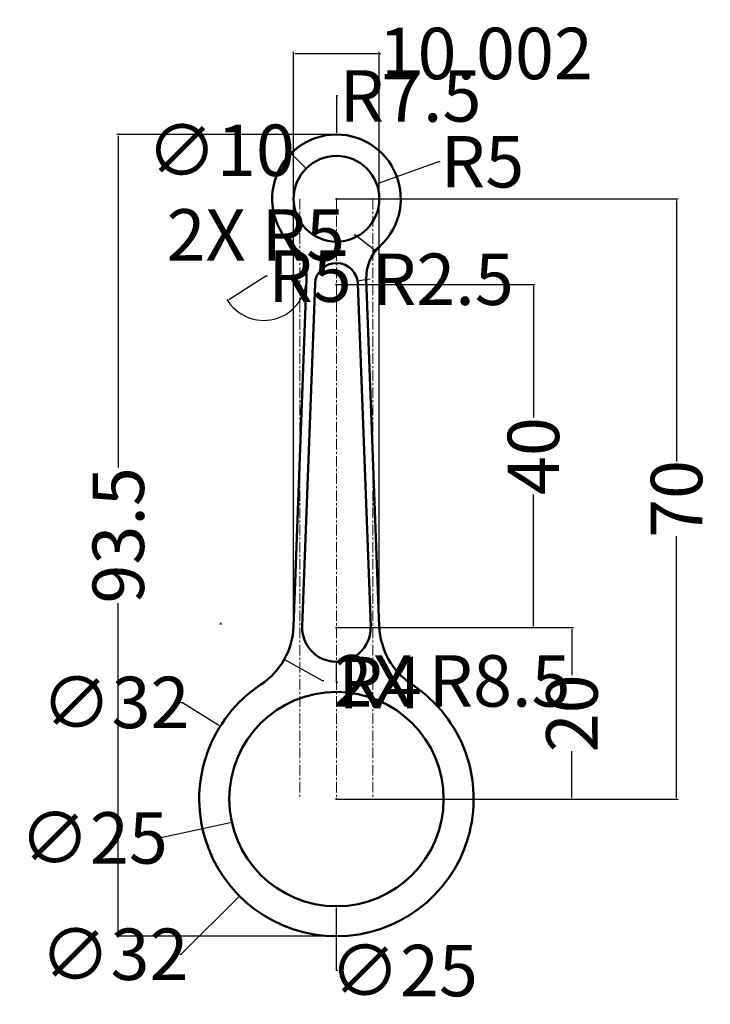
# Model space of a CAD drawing. Units: millimetres. Extents: x 20 to 101, y -5 to 109.
import ezdxf

# ---------------------------------------------------------------- set-up
doc = ezdxf.new("R2010")
doc.units = ezdxf.units.MM
doc.header["$MEASUREMENT"] = 0
doc.linetypes.add('CENTER', pattern=[2, 1.25, -0.25, 0.25, -0.25])
for name, color, linetype, lineweight in [('M-CNTR', 4, 'CENTER', 18), ('M-DIMS', 2, 'Continuous', 25), ('M-OUTL', 7, 'Continuous', 50)]:
    doc.layers.add(name, color=color, linetype=linetype, lineweight=lineweight)
doc.styles.get("Standard").update_dxf_attribs({"font": 'arial.ttf'})
doc.dimstyles.get("Standard").update_dxf_attribs({"dimtxt": 6, "dimasz": 0.18, "dimexe": 0.18, "dimexo": 0.0625, "dimgap": 0.09, "dimtad": 0, "dimtoh": 1, "dimdec": 0, "dimzin": 0, "dimdsep": 46, "dimtxsty": 'Standard', "dimcen": 0.09, "dimadec": 0, "dimazin": 0, "dimtfac": 1, "dimtdec": 0, "dimtofl": 0, "dimtmove": 0, "dimatfit": 3, "dimfxl": 1, "dimtolj": 1, "dimtzin": 0, "dimarcsym": 0})

# ---------------------------------------------------------------- blocks, each defined once
blk = doc.blocks.new('*D1')
at = {"layer": 'Defpoints', "color": 0, "transparency": 16777216}
for p in [(57.38, 78.56), (57.38, 38.56), (80.35, 38.56)]:
    blk.add_point(p, dxfattribs=at)
at = {"layer": 'M-DIMS', "color": 0, "lineweight": -2, "transparency": 16777216}
for p, q in [((57.44, 78.56), (80.53, 78.56)), ((80.35, 78.38), (80.35, 63.06)), ((80.35, 38.74), (80.35, 54.06)), ((57.44, 38.56), (80.53, 38.56))]:
    blk.add_line(p, q, dxfattribs=at)
at = {"layer": 'M-DIMS', "color": 0, "transparency": 16777216}
for points in [[(80.32, 78.38), (80.38, 78.38), (80.35, 78.56)], [(80.32, 38.74), (80.38, 38.74), (80.35, 38.56)]]:
    blk.add_solid(points, dxfattribs=at)
at = {"layer": 'M-DIMS', "color": 0, "transparency": 16777216, "insert": (80.35, 58.56), "char_height": 6, "attachment_point": 5, "rotation": 90}
blk.add_mtext('\\A1;40', dxfattribs=at)
blk = doc.blocks.new('*D2')
at = {"layer": 'Defpoints', "color": 0, "transparency": 16777216}
for p in [(57.38, 38.56), (57.38, 18.56), (84.84, 18.56)]:
    blk.add_point(p, dxfattribs=at)
at = {"layer": 'M-DIMS', "color": 0, "lineweight": -2, "transparency": 16777216}
for p, q in [((57.44, 38.56), (85.02, 38.56)), ((84.84, 38.38), (84.84, 32.99)), ((84.84, 18.74), (84.84, 24.13)), ((57.44, 18.56), (85.02, 18.56))]:
    blk.add_line(p, q, dxfattribs=at)
at = {"layer": 'M-DIMS', "color": 0, "transparency": 16777216}
for points in [[(84.81, 38.38), (84.87, 38.38), (84.84, 38.56)], [(84.81, 18.74), (84.87, 18.74), (84.84, 18.56)]]:
    blk.add_solid(points, dxfattribs=at)
at = {"layer": 'M-DIMS', "color": 0, "transparency": 16777216, "insert": (84.84, 28.56), "char_height": 6, "attachment_point": 5, "rotation": 90}
blk.add_mtext('\\A1;20', dxfattribs=at)
blk = doc.blocks.new('*D3')
at = {"layer": 'Defpoints', "color": 0, "transparency": 16777216}
for p in [(57.38, 88.56), (57.38, 18.56), (97.04, 18.56)]:
    blk.add_point(p, dxfattribs=at)
at = {"layer": 'M-DIMS', "color": 0, "lineweight": -2, "transparency": 16777216}
for p, q in [((57.44, 88.56), (97.22, 88.56)), ((97.04, 88.38), (97.04, 57.91)), ((97.04, 18.74), (97.04, 49.21)), ((57.44, 18.56), (97.22, 18.56))]:
    blk.add_line(p, q, dxfattribs=at)
at = {"layer": 'M-DIMS', "color": 0, "transparency": 16777216}
for points in [[(97.01, 88.38), (97.07, 88.38), (97.04, 88.56)], [(97.01, 18.74), (97.07, 18.74), (97.04, 18.56)]]:
    blk.add_solid(points, dxfattribs=at)
at = {"layer": 'M-DIMS', "color": 0, "transparency": 16777216, "insert": (97.04, 53.56), "char_height": 6, "attachment_point": 5, "rotation": 90}
blk.add_mtext('\\A1;70', dxfattribs=at)
blk = doc.blocks.new('*D4')
at = {"layer": 'Defpoints', "color": 0, "transparency": 16777216}
for p in [(48.9, 79.38), (44.7, 76.67)]:
    blk.add_point(p, dxfattribs=at)
at = {"layer": 'M-DIMS', "color": 0, "lineweight": -2, "transparency": 16777216}
for p, q in [((49.16, 79.54), (44.85, 76.77)), ((49.34, 79.54), (49.16, 79.54))]:
    blk.add_line(p, q, dxfattribs=at)
blk.add_arc((48.9, 79.38), 5, 210.6462, 357.1347, dxfattribs=at)
at = {"layer": 'M-DIMS', "color": 0, "transparency": 16777216}
blk.add_solid([(44.83, 76.8), (44.86, 76.75), (44.7, 76.67)], dxfattribs=at)
at = {"layer": 'M-DIMS', "color": 0, "transparency": 16777216, "insert": (54.29, 79.54), "char_height": 6, "attachment_point": 5}
blk.add_mtext('\\A1;R5', dxfattribs=at)
blk = doc.blocks.new('*D5')
at = {"layer": 'Defpoints', "color": 0, "transparency": 16777216}
for p in [(62.08, 90.27), (57.38, 88.56)]:
    blk.add_point(p, dxfattribs=at)
at = {"layer": 'M-DIMS', "color": 0, "lineweight": -2, "transparency": 16777216}
for p, q in [((69.28, 92.88), (62.25, 90.33)), ((69.46, 92.88), (69.28, 92.88)), ((57.29, 88.56), (57.47, 88.56)), ((57.38, 88.47), (57.38, 88.65))]:
    blk.add_line(p, q, dxfattribs=at)
at = {"layer": 'M-DIMS', "color": 0, "transparency": 16777216}
blk.add_solid([(62.24, 90.36), (62.26, 90.3), (62.08, 90.27)], dxfattribs=at)
at = {"layer": 'M-DIMS', "color": 0, "transparency": 16777216, "insert": (74.41, 92.88), "char_height": 6, "attachment_point": 5}
blk.add_mtext('\\A1;R5', dxfattribs=at)
blk = doc.blocks.new('*D6')
at = {"layer": 'Defpoints', "color": 0, "transparency": 16777216}
for p in [(43.83, 27.06), (70.94, 10.06)]:
    blk.add_point(p, dxfattribs=at)
at = {"layer": 'M-DIMS', "color": 0, "lineweight": -2, "transparency": 16777216}
for p, q in [((39.23, 29.83), (39.41, 29.83)), ((39.41, 29.83), (43.67, 27.16)), ((57.29, 18.56), (57.47, 18.56)), ((57.38, 18.47), (57.38, 18.65))]:
    blk.add_line(p, q, dxfattribs=at)
at = {"layer": 'M-DIMS', "color": 0, "transparency": 16777216}
blk.add_solid([(43.69, 27.18), (43.66, 27.13), (43.83, 27.06)], dxfattribs=at)
at = {"layer": 'M-DIMS', "color": 0, "transparency": 16777216, "insert": (31.61, 29.83), "char_height": 6, "attachment_point": 5}
blk.add_mtext('\\A1;∅32', dxfattribs=at)
blk = doc.blocks.new('*D7')
at = {"layer": 'Defpoints', "color": 0, "transparency": 16777216}
for p in [(69.59, 21.24), (45.17, 15.88)]:
    blk.add_point(p, dxfattribs=at)
at = {"layer": 'M-DIMS', "color": 0, "lineweight": -2, "transparency": 16777216}
for p, q in [((57.29, 18.56), (57.47, 18.56)), ((57.38, 18.47), (57.38, 18.65)), ((36.75, 14.03), (45, 15.84))]:
    blk.add_line(p, q, dxfattribs=at)
at = {"layer": 'M-DIMS', "color": 0, "transparency": 16777216}
blk.add_solid([(44.99, 15.87), (45, 15.81), (45.17, 15.88)], dxfattribs=at)
at = {"layer": 'M-DIMS', "color": 0, "transparency": 16777216, "insert": (29.08, 14.03), "char_height": 6, "attachment_point": 5}
blk.add_mtext('\\A1;∅25', dxfattribs=at)
blk = doc.blocks.new('*D8')
at = {"layer": 'Defpoints', "color": 0, "transparency": 16777216}
for p in [(31.94, 96.06), (57.38, 96.06), (57.38, 2.56)]:
    blk.add_point(p, dxfattribs=at)
at = {"layer": 'M-DIMS', "color": 0, "lineweight": -2, "transparency": 16777216}
for p, q in [((57.32, 96.06), (31.76, 96.06)), ((31.94, 95.88), (31.94, 57.22)), ((31.94, 2.74), (31.94, 41.41)), ((57.32, 2.56), (31.76, 2.56))]:
    blk.add_line(p, q, dxfattribs=at)
at = {"layer": 'M-DIMS', "color": 0, "transparency": 16777216}
for points in [[(31.91, 95.88), (31.97, 95.88), (31.94, 96.06)], [(31.91, 2.74), (31.97, 2.74), (31.94, 2.56)]]:
    blk.add_solid(points, dxfattribs=at)
at = {"layer": 'M-DIMS', "color": 0, "transparency": 16777216, "insert": (31.94, 49.31), "char_height": 6, "attachment_point": 5, "rotation": 90}
blk.add_mtext('\\A1;93.5', dxfattribs=at)
blk = doc.blocks.new('*D9')
at = {"layer": 'Defpoints', "color": 0, "transparency": 16777216}
for p in [(62.38, 105.51), (52.38, 38.69), (62.38, 38.69)]:
    blk.add_point(p, dxfattribs=at)
at = {"layer": 'M-DIMS', "color": 0, "lineweight": -2, "transparency": 16777216}
for p, q in [((52.38, 38.75), (52.38, 105.69)), ((62.38, 38.75), (62.38, 105.69)), ((52.56, 105.51), (62.2, 105.51)), ((62.38, 105.51), (62.56, 105.51))]:
    blk.add_line(p, q, dxfattribs=at)
at = {"layer": 'M-DIMS', "color": 0, "transparency": 16777216}
for points in [[(52.56, 105.54), (52.56, 105.48), (52.38, 105.51)], [(62.2, 105.54), (62.2, 105.48), (62.38, 105.51)]]:
    blk.add_solid(points, dxfattribs=at)
at = {"layer": 'M-DIMS', "color": 0, "transparency": 16777216, "insert": (74.79, 105.51), "char_height": 6, "attachment_point": 5}
blk.add_mtext('\\A1;10.002', dxfattribs=at)
blk = doc.blocks.new('*D10')
at = {"layer": 'Defpoints', "color": 0, "transparency": 16777216}
for p in [(68.69, 29.88), (46.07, 7.25)]:
    blk.add_point(p, dxfattribs=at)
at = {"layer": 'M-DIMS', "color": 0, "lineweight": -2, "transparency": 16777216}
for p, q in [((57.29, 18.56), (57.47, 18.56)), ((57.38, 18.47), (57.38, 18.65)), ((39.28, 0.46), (45.94, 7.12)), ((39.1, 0.46), (39.28, 0.46))]:
    blk.add_line(p, q, dxfattribs=at)
at = {"layer": 'M-DIMS', "color": 0, "transparency": 16777216}
blk.add_solid([(45.92, 7.14), (45.96, 7.1), (46.07, 7.25)], dxfattribs=at)
at = {"layer": 'M-DIMS', "color": 0, "transparency": 16777216, "insert": (31.48, 0.46), "char_height": 6, "attachment_point": 5}
blk.add_mtext('\\A1;∅32', dxfattribs=at)
blk = doc.blocks.new('*D11')
at = {"layer": 'Defpoints', "color": 0, "transparency": 16777216}
for p in [(57.38, 31.06), (57.38, 6.06)]:
    blk.add_point(p, dxfattribs=at)
at = {"layer": 'M-DIMS', "color": 0, "lineweight": -2, "transparency": 16777216}
for p, q in [((57.29, 18.56), (57.47, 18.56)), ((57.38, 18.47), (57.38, 18.65)), ((57.38, -1.44), (57.38, 5.88)), ((57.56, -1.44), (57.38, -1.44))]:
    blk.add_line(p, q, dxfattribs=at)
at = {"layer": 'M-DIMS', "color": 0, "transparency": 16777216}
blk.add_solid([(57.41, 5.88), (57.35, 5.88), (57.38, 6.06)], dxfattribs=at)
at = {"layer": 'M-DIMS', "color": 0, "transparency": 16777216, "insert": (65.24, -1.44), "char_height": 6, "attachment_point": 5}
blk.add_mtext('\\A1;∅25', dxfattribs=at)
blk = doc.blocks.new('*D12')
at = {"layer": 'Defpoints', "color": 0, "transparency": 16777216}
for p in [(43.89, 39.01), (51.29, 34.84)]:
    blk.add_point(p, dxfattribs=at)
at = {"layer": 'M-DIMS', "color": 0, "lineweight": -2, "transparency": 16777216}
for p, q in [((43.89, 38.92), (43.89, 39.1)), ((43.8, 39.01), (43.98, 39.01)), ((55.74, 32.34), (51.45, 34.75)), ((55.92, 32.34), (55.74, 32.34))]:
    blk.add_line(p, q, dxfattribs=at)
at = {"layer": 'M-DIMS', "color": 0, "transparency": 16777216}
blk.add_solid([(51.47, 34.78), (51.44, 34.73), (51.29, 34.84)], dxfattribs=at)
at = {"layer": 'M-DIMS', "color": 0, "transparency": 16777216, "insert": (70.86, 32.34), "char_height": 6, "attachment_point": 5}
blk.add_mtext('\\A1;2X R8.5', dxfattribs=at)
blk = doc.blocks.new('*D13')
at = {"layer": 'Defpoints', "color": 0, "transparency": 16777216}
for p in [(57.38, 96.06), (57.38, 88.56)]:
    blk.add_point(p, dxfattribs=at)
at = {"layer": 'M-DIMS', "color": 0, "lineweight": -2, "transparency": 16777216}
for p, q in [((57.56, 100.56), (57.38, 100.56)), ((57.38, 100.56), (57.38, 96.24)), ((57.29, 88.56), (57.47, 88.56)), ((57.38, 88.47), (57.38, 88.65))]:
    blk.add_line(p, q, dxfattribs=at)
at = {"layer": 'M-DIMS', "color": 0, "transparency": 16777216}
blk.add_solid([(57.35, 96.24), (57.41, 96.24), (57.38, 96.06)], dxfattribs=at)
at = {"layer": 'M-DIMS', "color": 0, "transparency": 16777216, "insert": (66.01, 100.56), "char_height": 6, "attachment_point": 5}
blk.add_mtext('\\A1;R7.5', dxfattribs=at)
blk = doc.blocks.new('*D14')
at = {"layer": 'Defpoints', "color": 0, "transparency": 16777216}
for p in [(53.85, 92.1), (60.92, 85.03)]:
    blk.add_point(p, dxfattribs=at)
at = {"layer": 'M-DIMS', "color": 0, "lineweight": -2, "transparency": 16777216}
for p, q in [((51.54, 94.22), (51.72, 94.22)), ((51.72, 94.22), (53.72, 92.23)), ((57.29, 88.56), (57.47, 88.56)), ((57.38, 88.47), (57.38, 88.65))]:
    blk.add_line(p, q, dxfattribs=at)
at = {"layer": 'M-DIMS', "color": 0, "transparency": 16777216}
blk.add_solid([(53.74, 92.25), (53.7, 92.2), (53.85, 92.1)], dxfattribs=at)
at = {"layer": 'M-DIMS', "color": 0, "transparency": 16777216, "insert": (43.9, 94.22), "char_height": 6, "attachment_point": 5}
blk.add_mtext('\\A1;∅10', dxfattribs=at)
blk = doc.blocks.new('*D15')
at = {"layer": 'Defpoints', "color": 0, "transparency": 16777216}
for p in [(61.94, 82.49), (65.86, 79.38)]:
    blk.add_point(p, dxfattribs=at)
at = {"layer": 'M-DIMS', "color": 0, "lineweight": -2, "transparency": 16777216}
for p, q in [((59.41, 84.35), (59.59, 84.35)), ((59.59, 84.35), (61.8, 82.6)), ((65.77, 79.38), (65.95, 79.38)), ((65.86, 79.29), (65.86, 79.47))]:
    blk.add_line(p, q, dxfattribs=at)
at = {"layer": 'M-DIMS', "color": 0, "transparency": 16777216}
blk.add_solid([(61.82, 82.62), (61.78, 82.58), (61.94, 82.49)], dxfattribs=at)
at = {"layer": 'M-DIMS', "color": 0, "transparency": 16777216, "insert": (47.97, 84.35), "char_height": 6, "attachment_point": 5}
blk.add_mtext('\\A1;2X R5', dxfattribs=at)
blk = doc.blocks.new('*D16')
at = {"layer": 'Defpoints', "color": 0, "transparency": 16777216}
for p in [(57.38, 38.56), (57.38, 34.56)]:
    blk.add_point(p, dxfattribs=at)
at = {"layer": 'M-DIMS', "color": 0, "lineweight": -2, "transparency": 16777216}
for p, q in [((57.29, 38.56), (57.47, 38.56)), ((57.38, 38.47), (57.38, 38.65)), ((57.38, 32.16), (57.38, 34.38)), ((57.56, 32.16), (57.38, 32.16))]:
    blk.add_line(p, q, dxfattribs=at)
at = {"layer": 'M-DIMS', "color": 0, "transparency": 16777216}
blk.add_solid([(57.41, 34.38), (57.35, 34.38), (57.38, 34.56)], dxfattribs=at)
at = {"layer": 'M-DIMS', "color": 0, "transparency": 16777216, "insert": (62.48, 32.16), "char_height": 6, "attachment_point": 5}
blk.add_mtext('\\A1;R4', dxfattribs=at)
blk = doc.blocks.new('*D17')
at = {"layer": 'Defpoints', "color": 0, "transparency": 16777216}
for p in [(57.38, 78.56), (59.85, 78.95)]:
    blk.add_point(p, dxfattribs=at)
at = {"layer": 'M-DIMS', "color": 0, "lineweight": -2, "transparency": 16777216}
for p, q in [((57.29, 78.56), (57.47, 78.56)), ((57.38, 78.47), (57.38, 78.65)), ((61.33, 79.18), (60.03, 78.98))]:
    blk.add_line(p, q, dxfattribs=at)
at = {"layer": 'M-DIMS', "color": 0, "transparency": 16777216}
blk.add_solid([(60.02, 79.01), (60.03, 78.95), (59.85, 78.95)], dxfattribs=at)
at = {"layer": 'M-DIMS', "color": 0, "transparency": 16777216, "insert": (69.78, 79.18), "char_height": 6, "attachment_point": 5}
blk.add_mtext('\\A1;R2.5', dxfattribs=at)

msp = doc.modelspace()

# ---------------------------------------------------------------- linework, layer by layer
at = {"layer": 'M-CNTR'}
for p, q in [((53.1307, 88.5622), (53.1307, 18.5622)), ((57.3807, 88.5622), (57.3807, 18.5622)), ((61.6307, 88.5622), (61.6307, 18.5622))]:
    msp.add_line(p, q, dxfattribs=at)
at = {"layer": 'M-OUTL'}
for p, q in [((53.8995, 79.1889), (52.3798, 38.6918)), ((54.8825, 78.6559), (53.3836, 38.7122)), ((59.879, 78.6559), (61.3779, 38.7122)), ((60.862, 79.1889), (62.3817, 38.6918))]:
    msp.add_line(p, q, dxfattribs=at)
for centre, radius in [((57.3807, 88.5622), 5), ((57.3807, 18.5622), 12.5)]:
    msp.add_circle(centre, radius, dxfattribs=at)
for centre, radius, start, end in [((57.3807, 88.5622), 7.5, 304.518108, 235.481892), ((48.903, 79.3764), 5, 357.850904, 47.295513), ((65.8585, 79.3764), 5, 132.704487, 182.149096), ((57.3807, 78.5622), 2.5, 0, 177.850904), ((43.8858, 39.0106), 8.5, 303.422933, 357.850904), ((57.3807, 38.5622), 4, 177.850904, 2.149096), ((70.8757, 39.0106), 8.5, 182.149096, 236.577067), ((57.3807, 18.5622), 16, 123.422933, 56.577067)]:
    msp.add_arc(centre, radius, start, end, dxfattribs=at)

# ---------------------------------------------------------------- dimensions: what is measured, and where the dimension line sits
at = {"layer": 'M-DIMS'}
dim = msp.add_linear_dim(base=(62.3817, 105.5122), p1=(52.3798, 38.6918), p2=(62.3817, 38.6918), dimstyle='Standard', override={"dimdec": 3, "dimlfac": 1, "dimrnd": 0, "dimzin": 0, "dimdsep": 46, "dimlunit": 2}, dxfattribs=at)
dim.commit()
dim.dimension.update_dxf_attribs({"geometry": '*D9', "text_midpoint": (74.7929, 105.5122)})
for center, mpoint, override, picture, middle in [((57.3807, 88.5622), (57.381, 96.0622), {"dimdec": 1, "dimlfac": 1, "dimrnd": 0, "dimzin": 0, "dimdsep": 46, "dimlunit": 2}, '*D13', (66.0065, 100.5622)), ((57.3807, 88.5622), (62.0805, 90.2689), {"dimclrd": 0, "dimclre": 0, "dimclrt": 0}, '*D5', (74.4096, 92.8831)), ((48.903, 79.3764), (44.6959, 76.6746), {"dimclrd": 0, "dimclre": 0, "dimclrt": 0}, '*D4', (54.2942, 79.544)), ((57.3807, 78.5622), (59.8505, 78.9501), {"dimdec": 1, "dimlfac": 1, "dimrnd": 0, "dimzin": 0, "dimdsep": 46, "dimlunit": 2}, '*D17', (61.3323, 79.1828)), ((57.3807, 38.5622), (57.381, 34.5622), {"dimdec": 0, "dimlfac": 1, "dimrnd": 0, "dimzin": 0, "dimdsep": 46, "dimlunit": 2}, '*D16', (62.4765, 32.1622))]:
    dim = msp.add_radius_dim(center=center, mpoint=mpoint, dimstyle='Standard', override=override, dxfattribs=at)
    dim.commit()
    dim.dimension.update_dxf_attribs({"geometry": picture, "text_midpoint": middle, "dimtype": 164})
for p1, p2, override, picture, middle in [((60.9157, 85.0261), (53.8457, 92.0983), {"dimdec": 0, "dimlfac": 1, "dimrnd": 0, "dimzin": 0, "dimdsep": 46, "dimlunit": 2}, '*D14', (43.9036, 94.2199)), ((70.9357, 10.0615), (43.8257, 27.0629), {"dimclrd": 0, "dimclre": 0, "dimclrt": 0}, '*D6', (31.6087, 29.8325)), ((57.3805, 31.0622), (57.381, 6.0622), {"dimdec": 0, "dimlfac": 1, "dimrnd": 0, "dimzin": 0, "dimdsep": 46, "dimlunit": 2}, '*D11', (65.2351, -1.4378)), ((68.6947, 29.8756), (46.0668, 7.2488), {"dimdec": 0, "dimlfac": 1, "dimrnd": 0, "dimzin": 0, "dimdsep": 46, "dimlunit": 2}, '*D10', (31.4777, 0.4607)), ((69.59, 21.2426), (45.1715, 15.8818), {"dimclrd": 0, "dimclre": 0, "dimclrt": 0}, '*D7', (36.7515, 14.0332))]:
    dim = msp.add_diameter_dim_2p(p1=p1, p2=p2, dimstyle='Standard', override=override, dxfattribs=at)
    dim.commit()
    dim.dimension.update_dxf_attribs({"geometry": picture, "text_midpoint": middle, "dimtype": 163})
for base, p1, p2, override, picture, middle in [((31.9377, 96.0622), (57.3807, 2.5622), (57.3807, 96.0622), {"dimdec": 1, "dimlfac": 1, "dimrnd": 0, "dimzin": 0, "dimdsep": 46, "dimlunit": 2}, '*D8', (31.9377, 49.3122)), ((97.0433, 18.5622), (57.3807, 88.5622), (57.3807, 18.5622), {"dimclrd": 0, "dimclre": 0, "dimclrt": 0}, '*D3', (97.0433, 53.5622)), ((80.3503, 38.5622), (57.3807, 78.5622), (57.3807, 38.5622), {"dimclrd": 0, "dimclre": 0, "dimclrt": 0}, '*D1', (80.3503, 58.5622)), ((84.8446, 18.5622), (57.3807, 38.5622), (57.3807, 18.5622), {"dimclrd": 0, "dimclre": 0, "dimclrt": 0}, '*D2', (84.8446, 28.5622))]:
    dim = msp.add_linear_dim(base=base, p1=p1, p2=p2, angle=90, dimstyle='Standard', override=override, dxfattribs=at)
    dim.commit()
    dim.dimension.update_dxf_attribs({"geometry": picture, "text_midpoint": middle})
for center, mpoint, override, picture, middle in [((65.8585, 79.3764), (61.9436, 82.4867), {"dimdec": 0, "dimlfac": 1, "dimrnd": 0, "dimzin": 0, "dimdsep": 46, "dimlunit": 2}, '*D15', (47.9672, 84.3528)), ((43.8858, 39.0106), (51.294, 34.843), {"dimdec": 1, "dimlfac": 1, "dimrnd": 0, "dimzin": 0, "dimdsep": 46, "dimlunit": 2}, '*D12', (70.8616, 32.3425))]:
    dim = msp.add_radius_dim(center=center, mpoint=mpoint, text='2X <>', dimstyle='Standard', override=override, dxfattribs=at)
    dim.commit()
    dim.dimension.update_dxf_attribs({"geometry": picture, "text_midpoint": middle, "dimtype": 164})

doc.saveas('drawing.dxf')
